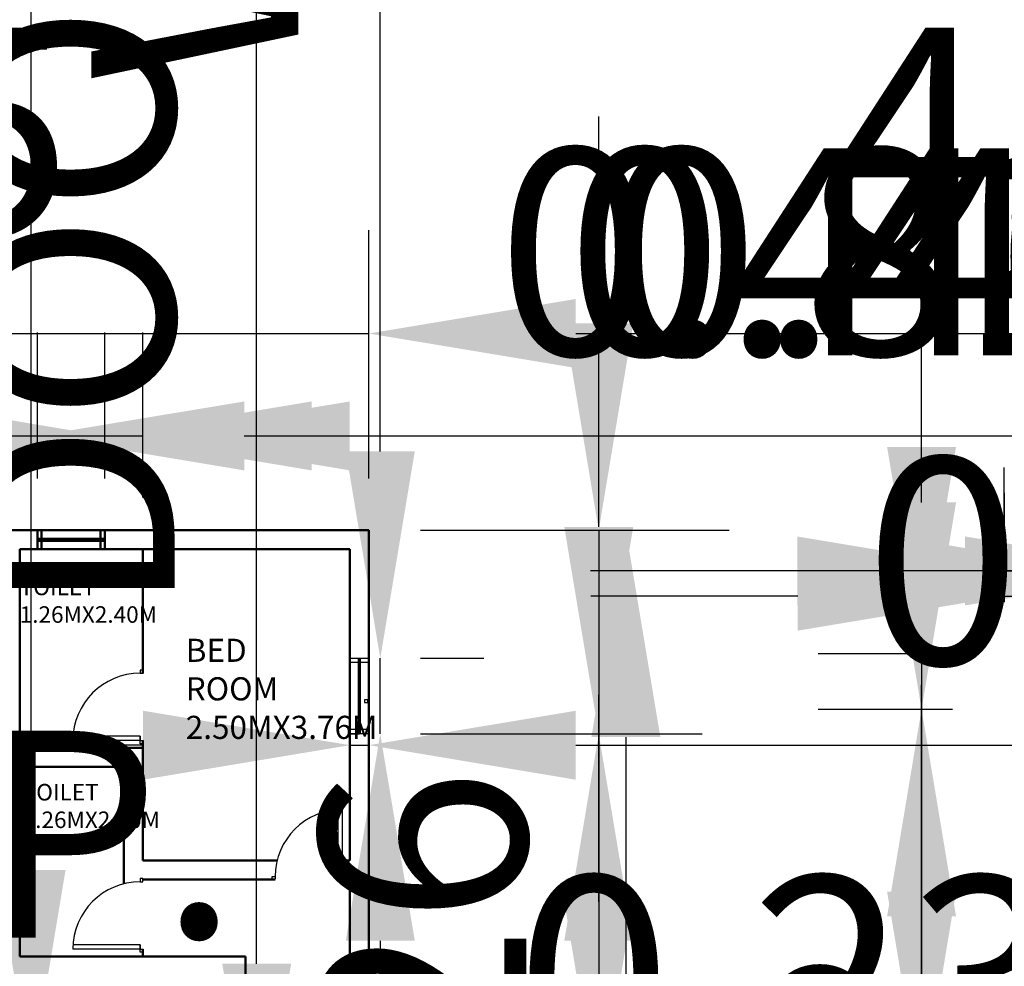
# Model space of a CAD drawing. Units: metres. Extents: x 782 to 1487, y 1262 to 7446.
# Tile 17 of 25: x 828.19 to 840.09, y 1302.06 to 1313.5. Entities that reach past the tile are written whole.
import ezdxf

# ---------------------------------------------------------------- set-up
doc = ezdxf.new("R2010")
doc.units = ezdxf.units.M
for name, color, linetype, lineweight in [('A-ANNO-DIMS', 2, 'Continuous', 18), ('A-AREA-IDEN', 3, 'Continuous', 18), ('A-DOOR', 4, 'Continuous', 25), ('A-GLAZ', 4, 'Continuous', 25), ('A-WALL', 7, 'Continuous', 50)]:
    doc.layers.add(name, color=color, linetype=linetype, lineweight=lineweight)
doc.styles.get("Standard").update_dxf_attribs({"font": 'arial.ttf'})
doc.dimstyles.new('ISO-25', dxfattribs={"dimtxt": 2.5, "dimasz": 2.5, "dimexe": 1.25, "dimexo": 0.625, "dimtad": 1, "dimtxsty": 'Standard', "dimcen": 2.5, "dimadec": 0, "dimazin": 0, "dimtfac": 1, "dimtmove": 0, "dimatfit": 3, "dimfxl": 1, "dimarcsym": 0})

# ---------------------------------------------------------------- blocks, each defined once
blk = doc.blocks.new('*D5')
at = {"layer": 'A-ANNO-DIMS', "color": 0, "lineweight": -2, "transparency": 16777216}
for p, q in [((812.13, 1307.952), (812.13, 1310.955)), ((816.58, 1307.952), (816.58, 1310.955)), ((809.63, 1309.705), (807.13, 1309.705)), ((812.13, 1309.705), (816.58, 1309.705)), ((819.08, 1309.705), (829.443, 1309.705))]:
    blk.add_line(p, q, dxfattribs=at)
at = {"layer": 'A-ANNO-DIMS', "color": 0, "transparency": 16777216}
for points in [[(809.63, 1310.122), (809.63, 1309.289), (812.13, 1309.705)], [(819.08, 1310.122), (819.08, 1309.289), (816.58, 1309.705)]]:
    blk.add_solid(points, dxfattribs=at)
at = {"layer": 'Defpoints', "color": 0, "transparency": 16777216}
for p in [(816.58, 1309.705), (812.13, 1307.327), (816.58, 1307.327)]:
    blk.add_point(p, dxfattribs=at)
at = {"layer": 'A-ANNO-DIMS', "color": 0, "transparency": 16777216, "insert": (825.512, 1311.828), "char_height": 2.5, "attachment_point": 5}
blk.add_mtext('4,45', dxfattribs=at)
blk = doc.blocks.new('*D6')
at = {"layer": 'A-ANNO-DIMS', "color": 0, "lineweight": -2, "transparency": 16777216}
for p, q in [((833.037, 1307.327), (836.768, 1307.327)), ((835.518, 1304.827), (835.518, 1295.567)), ((833.037, 1293.067), (836.768, 1293.067))]:
    blk.add_line(p, q, dxfattribs=at)
at = {"layer": 'A-ANNO-DIMS', "color": 0, "transparency": 16777216}
for points in [[(835.102, 1304.827), (835.935, 1304.827), (835.518, 1307.327)], [(835.102, 1295.567), (835.935, 1295.567), (835.518, 1293.067)]]:
    blk.add_solid(points, dxfattribs=at)
at = {"layer": 'Defpoints', "color": 0, "transparency": 16777216}
for p in [(832.412, 1307.327), (832.412, 1293.067), (835.518, 1293.067)]:
    blk.add_point(p, dxfattribs=at)
at = {"layer": 'A-ANNO-DIMS', "color": 0, "transparency": 16777216, "insert": (833.391, 1300.197), "char_height": 2.5, "attachment_point": 5, "rotation": 90}
blk.add_mtext('14,26', dxfattribs=at)
blk = doc.blocks.new('*D7')
at = {"layer": 'A-ANNO-DIMS', "color": 0, "lineweight": -2, "transparency": 16777216}
for p, q in [((827.962, 1307.952), (827.962, 1310.955)), ((832.412, 1307.952), (832.412, 1310.955)), ((825.462, 1309.705), (822.962, 1309.705)), ((827.962, 1309.705), (832.412, 1309.705)), ((834.912, 1309.705), (845.276, 1309.705))]:
    blk.add_line(p, q, dxfattribs=at)
at = {"layer": 'A-ANNO-DIMS', "color": 0, "transparency": 16777216}
for points in [[(825.462, 1310.122), (825.462, 1309.289), (827.962, 1309.705)], [(834.912, 1310.122), (834.912, 1309.289), (832.412, 1309.705)]]:
    blk.add_solid(points, dxfattribs=at)
at = {"layer": 'Defpoints', "color": 0, "transparency": 16777216}
for p in [(832.412, 1309.705), (827.962, 1307.327), (832.412, 1307.327)]:
    blk.add_point(p, dxfattribs=at)
at = {"layer": 'A-ANNO-DIMS', "color": 0, "transparency": 16777216, "insert": (841.344, 1311.828), "char_height": 2.5, "attachment_point": 5}
blk.add_mtext('4,45', dxfattribs=at)
blk = doc.blocks.new('*D9')
at = {"layer": 'A-ANNO-DIMS', "color": 0, "lineweight": -2, "transparency": 16777216}
for p, q in [((840.095, 1306.46), (840.095, 1307.78)), ((844.185, 1306.46), (844.185, 1307.78)), ((837.595, 1306.53), (835.095, 1306.53)), ((840.095, 1306.53), (844.185, 1306.53)), ((846.685, 1306.53), (857.034, 1306.53))]:
    blk.add_line(p, q, dxfattribs=at)
at = {"layer": 'A-ANNO-DIMS', "color": 0, "transparency": 16777216}
for points in [[(837.595, 1306.947), (837.595, 1306.114), (840.095, 1306.53)], [(846.685, 1306.947), (846.685, 1306.114), (844.185, 1306.53)]]:
    blk.add_solid(points, dxfattribs=at)
at = {"layer": 'Defpoints', "color": 0, "transparency": 16777216}
for p in [(844.185, 1306.53), (840.095, 1305.835), (844.185, 1305.835)]:
    blk.add_point(p, dxfattribs=at)
at = {"layer": 'A-ANNO-DIMS', "color": 0, "transparency": 16777216, "insert": (853.11, 1308.658), "char_height": 2.5, "attachment_point": 5}
blk.add_mtext('4,09', dxfattribs=at)
blk = doc.blocks.new('DOOR-810')
for p, q in [((0.813, 0.089), (0, 0.089)), ((0.813, 0.038), (0.813, 0.089))]:
    blk.add_line(p, q)
for points in [[(0.813, 0.851), (0.846, 0.851), (0.846, 0.89), (0.813, 0.89)], [(0.813, 0.038), (0.847, 0.038), (0.847, 0), (0.813, 0)]]:
    blk.add_lwpolyline(points, close=True)
blk.add_lwpolyline([(0.813, 0.089), (0.813, 0.038), (0, 0.038)])
blk.add_arc((0.813, 0.038), 0.813, 90, 180)
blk = doc.blocks.new('DOOR-810-C')
for p, q in [((0.801, 0.034), (0.801, 0.847)), ((0.851, 0.034), (0.801, 0.034))]:
    blk.add_line(p, q)
blk.add_lwpolyline([(0.801, 0.034), (0.851, 0.034), (0.851, 0.847)])
for points in [[(0.039, 0.034), (0.039, 0.002), (0, 0.002), (0, 0.034)], [(0.851, 0.034), (0.851, 0), (0.889, 0), (0.889, 0.034)]]:
    blk.add_lwpolyline(points, close=True)
blk.add_arc((0.851, 0.034), 0.813, 90, 180)
blk = doc.blocks.new('WIN-900-B')
for p, q in [((0, 0), (0, 0.914)), ((0, 0.914), (0.23, 0.914)), ((0.23, 0.863), (0, 0.863)), ((0.103, 0), (0.103, 0.914)), ((0.115, 0), (0.115, 0.914)), ((0.128, 0), (0.128, 0.914)), ((0.23, 0.914), (0.23, 0)), ((0.23, 0.914), (0.23, 0.863)), ((0.23, 0.051), (0, 0.051)), ((0.23, 0), (0.23, 0.051)), ((0.23, 0), (0, 0)), ((0, 0), (0.115, 0))]:
    blk.add_line(p, q)
blk.add_lwpolyline([(0.215, 0.379), (0.215, 0.412), (0.176, 0.412), (0.176, 0.379)], close=True)
blk = doc.blocks.new('*D20')
at = {"layer": 'A-ANNO-DIMS', "color": 0, "lineweight": -2, "transparency": 16777216}
for p, q in [((831.056, 1302.088), (831.056, 1337.678)), ((831.056, 1298.698), (831.056, 1299.588)), ((831.548, 1299.588), (832.306, 1299.588)), ((831.548, 1298.698), (832.306, 1298.698)), ((831.056, 1296.198), (831.056, 1293.698))]:
    blk.add_line(p, q, dxfattribs=at)
at = {"layer": 'A-ANNO-DIMS', "color": 0, "transparency": 16777216}
for points in [[(830.64, 1302.088), (831.473, 1302.088), (831.056, 1299.588)], [(830.64, 1296.198), (831.473, 1296.198), (831.056, 1298.698)]]:
    blk.add_solid(points, dxfattribs=at)
at = {"layer": 'Defpoints', "color": 0, "transparency": 16777216}
for p in [(830.923, 1299.588), (831.056, 1299.588), (830.923, 1298.698)]:
    blk.add_point(p, dxfattribs=at)
at = {"layer": 'A-ANNO-DIMS', "color": 0, "transparency": 16777216, "insert": (829.138, 1321.133), "char_height": 2.5, "attachment_point": 5, "rotation": 90}
blk.add_mtext('DOOR D1 0.89 TYP.', dxfattribs=at)
blk = doc.blocks.new('*D21')
at = {"layer": 'A-ANNO-DIMS', "color": 0, "lineweight": -2, "transparency": 16777216}
for p, q in [((827.576, 1298.565), (825.076, 1298.565)), ((830.076, 1298.565), (830.923, 1298.565)), ((833.423, 1298.565), (852.255, 1298.565)), ((830.076, 1298.073), (830.076, 1297.315)), ((830.923, 1298.073), (830.923, 1297.315))]:
    blk.add_line(p, q, dxfattribs=at)
at = {"layer": 'A-ANNO-DIMS', "color": 0, "transparency": 16777216}
for points in [[(827.576, 1298.981), (827.576, 1298.148), (830.076, 1298.565)], [(833.423, 1298.981), (833.423, 1298.148), (830.923, 1298.565)]]:
    blk.add_solid(points, dxfattribs=at)
at = {"layer": 'Defpoints', "color": 0, "transparency": 16777216}
for p in [(830.076, 1298.698), (830.923, 1298.698), (830.923, 1298.565)]:
    blk.add_point(p, dxfattribs=at)
at = {"layer": 'A-ANNO-DIMS', "color": 0, "transparency": 16777216, "insert": (844.089, 1300.466), "char_height": 2.5, "attachment_point": 5}
blk.add_mtext('0.85 TYP.', dxfattribs=at)
blk = doc.blocks.new('*D24')
at = {"layer": 'A-ANNO-DIMS', "color": 0, "lineweight": -2, "transparency": 16777216}
for p, q in [((811.209, 1294.423), (808.709, 1294.423)), ((813.709, 1294.423), (814.559, 1294.423)), ((817.059, 1294.423), (852.649, 1294.423)), ((813.709, 1293.926), (813.709, 1293.173)), ((814.559, 1293.926), (814.559, 1293.173))]:
    blk.add_line(p, q, dxfattribs=at)
at = {"layer": 'A-ANNO-DIMS', "color": 0, "transparency": 16777216}
for points in [[(811.209, 1294.84), (811.209, 1294.006), (813.709, 1294.423)], [(817.059, 1294.84), (817.059, 1294.006), (814.559, 1294.423)]]:
    blk.add_solid(points, dxfattribs=at)
at = {"layer": 'Defpoints', "color": 0, "transparency": 16777216}
for p in [(813.709, 1294.551), (814.559, 1294.551), (814.559, 1294.423)]:
    blk.add_point(p, dxfattribs=at)
at = {"layer": 'A-ANNO-DIMS', "color": 0, "transparency": 16777216, "insert": (836.104, 1296.342), "char_height": 2.5, "attachment_point": 5}
blk.add_mtext('DOOR D2 0.85 TYP.', dxfattribs=at)
blk = doc.blocks.new('*D26')
at = {"layer": 'A-ANNO-DIMS', "color": 0, "lineweight": -2, "transparency": 16777216}
for p, q in [((828.33, 1303.223), (828.33, 1342.718)), ((828.33, 1299.809), (828.33, 1300.723)), ((828.818, 1300.723), (829.58, 1300.723)), ((828.818, 1299.809), (829.58, 1299.809)), ((828.33, 1297.309), (828.33, 1294.809))]:
    blk.add_line(p, q, dxfattribs=at)
at = {"layer": 'A-ANNO-DIMS', "color": 0, "transparency": 16777216}
for points in [[(827.913, 1303.223), (828.747, 1303.223), (828.33, 1300.723)], [(827.913, 1297.309), (828.747, 1297.309), (828.33, 1299.809)]]:
    blk.add_solid(points, dxfattribs=at)
at = {"layer": 'Defpoints', "color": 0, "transparency": 16777216}
for p in [(828.193, 1300.723), (828.33, 1300.723), (828.193, 1299.809)]:
    blk.add_point(p, dxfattribs=at)
at = {"layer": 'A-ANNO-DIMS', "color": 0, "transparency": 16777216, "insert": (826.412, 1324.22), "char_height": 2.5, "attachment_point": 5, "rotation": 90}
blk.add_mtext('WINDOW W 0.91 TYP.', dxfattribs=at)
blk = doc.blocks.new('*D27')
at = {"layer": 'A-ANNO-DIMS', "color": 0, "lineweight": -2, "transparency": 16777216}
for p, q in [((825.463, 1299.672), (822.963, 1299.672)), ((827.963, 1299.672), (828.193, 1299.672)), ((830.693, 1299.672), (849.525, 1299.672)), ((827.963, 1299.184), (827.963, 1298.422)), ((828.193, 1299.184), (828.193, 1298.422))]:
    blk.add_line(p, q, dxfattribs=at)
at = {"layer": 'A-ANNO-DIMS', "color": 0, "transparency": 16777216}
for points in [[(825.463, 1300.088), (825.463, 1299.255), (827.963, 1299.672)], [(830.693, 1300.088), (830.693, 1299.255), (828.193, 1299.672)]]:
    blk.add_solid(points, dxfattribs=at)
at = {"layer": 'Defpoints', "color": 0, "transparency": 16777216}
for p in [(827.963, 1299.809), (828.193, 1299.809), (828.193, 1299.672)]:
    blk.add_point(p, dxfattribs=at)
at = {"layer": 'A-ANNO-DIMS', "color": 0, "transparency": 16777216, "insert": (841.359, 1301.574), "char_height": 2.5, "attachment_point": 5}
blk.add_mtext('0.23 TYP.', dxfattribs=at)
blk = doc.blocks.new('*D28')
at = {"layer": 'A-ANNO-DIMS', "color": 0, "lineweight": -2, "transparency": 16777216}
for p, q in [((832.55, 1308.281), (832.55, 1349.718)), ((832.55, 1304.867), (832.55, 1305.781)), ((833.038, 1305.781), (833.8, 1305.781)), ((833.038, 1304.867), (833.8, 1304.867)), ((832.55, 1302.367), (832.55, 1299.867))]:
    blk.add_line(p, q, dxfattribs=at)
at = {"layer": 'A-ANNO-DIMS', "color": 0, "transparency": 16777216}
for points in [[(832.134, 1308.281), (832.967, 1308.281), (832.55, 1305.781)], [(832.134, 1302.367), (832.967, 1302.367), (832.55, 1304.867)]]:
    blk.add_solid(points, dxfattribs=at)
at = {"layer": 'Defpoints', "color": 0, "transparency": 16777216}
for p in [(832.413, 1305.781), (832.55, 1305.781), (832.413, 1304.867)]:
    blk.add_point(p, dxfattribs=at)
at = {"layer": 'A-ANNO-DIMS', "color": 0, "transparency": 16777216, "insert": (830.632, 1330.25), "char_height": 2.5, "attachment_point": 5, "rotation": 90}
blk.add_mtext('WINDOW W1 0.91 TYP.', dxfattribs=at)
blk = doc.blocks.new('*D29')
at = {"layer": 'A-ANNO-DIMS', "color": 0, "lineweight": -2, "transparency": 16777216}
for p, q in [((829.683, 1304.73), (827.183, 1304.73)), ((832.183, 1304.73), (832.413, 1304.73)), ((834.913, 1304.73), (853.745, 1304.73)), ((832.183, 1304.242), (832.183, 1303.48)), ((832.413, 1304.242), (832.413, 1303.48))]:
    blk.add_line(p, q, dxfattribs=at)
at = {"layer": 'A-ANNO-DIMS', "color": 0, "transparency": 16777216}
for points in [[(829.683, 1305.146), (829.683, 1304.313), (832.183, 1304.73)], [(834.913, 1305.146), (834.913, 1304.313), (832.413, 1304.73)]]:
    blk.add_solid(points, dxfattribs=at)
at = {"layer": 'Defpoints', "color": 0, "transparency": 16777216}
for p in [(832.183, 1304.867), (832.413, 1304.867), (832.413, 1304.73)]:
    blk.add_point(p, dxfattribs=at)
at = {"layer": 'A-ANNO-DIMS', "color": 0, "transparency": 16777216, "insert": (845.579, 1306.632), "char_height": 2.5, "attachment_point": 5}
blk.add_mtext('0.23 TYP.', dxfattribs=at)
blk = doc.blocks.new('*D30')
at = {"layer": 'A-ANNO-DIMS', "color": 0, "lineweight": -2, "transparency": 16777216}
for p, q in [((792.059, 1301.411), (789.559, 1301.411)), ((794.559, 1301.411), (794.946, 1301.411)), ((797.446, 1301.411), (832.354, 1301.411)), ((794.559, 1300.844), (794.559, 1300.161)), ((794.946, 1300.844), (794.946, 1300.161))]:
    blk.add_line(p, q, dxfattribs=at)
at = {"layer": 'A-ANNO-DIMS', "color": 0, "transparency": 16777216}
for points in [[(792.059, 1301.827), (792.059, 1300.994), (794.559, 1301.411)], [(797.446, 1301.827), (797.446, 1300.994), (794.946, 1301.411)]]:
    blk.add_solid(points, dxfattribs=at)
at = {"layer": 'Defpoints', "color": 0, "transparency": 16777216}
for p in [(794.559, 1301.469), (794.946, 1301.469), (794.946, 1301.411)]:
    blk.add_point(p, dxfattribs=at)
at = {"layer": 'A-ANNO-DIMS', "color": 0, "transparency": 16777216, "insert": (816.15, 1303.33), "char_height": 2.5, "attachment_point": 5}
blk.add_mtext('COLUMN 0.39 TYP.', dxfattribs=at)
blk = doc.blocks.new('*D87')
at = {"layer": 'A-ANNO-DIMS', "color": 0, "lineweight": -2, "transparency": 16777216}
for p, q in [((835.19, 1309.827), (835.19, 1312.327)), ((833.037, 1307.327), (836.44, 1307.327)), ((835.19, 1307.327), (835.19, 1304.867)), ((833.038, 1304.867), (836.44, 1304.867)), ((835.19, 1302.367), (835.19, 1292.082))]:
    blk.add_line(p, q, dxfattribs=at)
at = {"layer": 'A-ANNO-DIMS', "color": 0, "transparency": 16777216}
for points in [[(834.774, 1309.827), (835.607, 1309.827), (835.19, 1307.327)], [(834.774, 1302.367), (835.607, 1302.367), (835.19, 1304.867)]]:
    blk.add_solid(points, dxfattribs=at)
at = {"layer": 'Defpoints', "color": 0, "transparency": 16777216}
for p in [(832.412, 1307.327), (832.413, 1304.867), (835.19, 1304.867)]:
    blk.add_point(p, dxfattribs=at)
at = {"layer": 'A-ANNO-DIMS', "color": 0, "transparency": 16777216, "insert": (833.289, 1295.974), "char_height": 2.5, "attachment_point": 5, "rotation": 90}
blk.add_mtext('2.46', dxfattribs=at)
blk = doc.blocks.new('*D88')
at = {"layer": 'A-ANNO-DIMS', "color": 0, "lineweight": -2, "transparency": 16777216}
for p, q in [((835.19, 1307.367), (835.19, 1309.867)), ((833.038, 1304.867), (836.44, 1304.867)), ((835.19, 1304.867), (835.19, 1300.338)), ((833.038, 1300.338), (836.44, 1300.338)), ((835.19, 1297.838), (835.19, 1285.546))]:
    blk.add_line(p, q, dxfattribs=at)
at = {"layer": 'A-ANNO-DIMS', "color": 0, "transparency": 16777216}
for points in [[(834.774, 1307.367), (835.607, 1307.367), (835.19, 1304.867)], [(834.774, 1297.838), (835.607, 1297.838), (835.19, 1300.338)]]:
    blk.add_solid(points, dxfattribs=at)
at = {"layer": 'Defpoints', "color": 0, "transparency": 16777216}
for p in [(832.413, 1304.867), (832.413, 1300.338), (835.19, 1300.338)]:
    blk.add_point(p, dxfattribs=at)
at = {"layer": 'A-ANNO-DIMS', "color": 0, "transparency": 16777216, "insert": (833.289, 1290.442), "char_height": 2.5, "attachment_point": 5, "rotation": 90}
blk.add_mtext('4.529', dxfattribs=at)
blk = doc.blocks.new('*D89')
at = {"layer": 'A-ANNO-DIMS', "color": 0, "lineweight": -2, "transparency": 16777216}
for p, q in [((835.19, 1302.838), (835.19, 1305.338)), ((833.038, 1300.338), (836.44, 1300.338)), ((835.19, 1300.338), (835.19, 1296.196)), ((833.037, 1296.196), (836.44, 1296.196)), ((835.19, 1293.696), (835.19, 1281.435))]:
    blk.add_line(p, q, dxfattribs=at)
at = {"layer": 'A-ANNO-DIMS', "color": 0, "transparency": 16777216}
for points in [[(834.774, 1302.838), (835.607, 1302.838), (835.19, 1300.338)], [(834.774, 1293.696), (835.607, 1293.696), (835.19, 1296.196)]]:
    blk.add_solid(points, dxfattribs=at)
at = {"layer": 'Defpoints', "color": 0, "transparency": 16777216}
for p in [(832.413, 1300.338), (832.412, 1296.196), (835.19, 1296.196)]:
    blk.add_point(p, dxfattribs=at)
at = {"layer": 'A-ANNO-DIMS', "color": 0, "transparency": 16777216, "insert": (833.31, 1286.315), "char_height": 2.5, "attachment_point": 5, "rotation": 90}
blk.add_mtext('4.142', dxfattribs=at)
blk = doc.blocks.new('*D94')
at = {"layer": 'A-ANNO-DIMS', "color": 0, "lineweight": -2, "transparency": 16777216}
for p, q in [((827.962, 1307.952), (827.962, 1309.718)), ((828.406, 1307.953), (828.406, 1309.718)), ((825.462, 1308.468), (822.962, 1308.468)), ((827.962, 1308.468), (828.406, 1308.468)), ((830.906, 1308.468), (841.139, 1308.468))]:
    blk.add_line(p, q, dxfattribs=at)
at = {"layer": 'A-ANNO-DIMS', "color": 0, "transparency": 16777216}
for points in [[(825.462, 1308.884), (825.462, 1308.051), (827.962, 1308.468)], [(830.906, 1308.884), (830.906, 1308.051), (828.406, 1308.468)]]:
    blk.add_solid(points, dxfattribs=at)
at = {"layer": 'Defpoints', "color": 0, "transparency": 16777216}
for p in [(828.406, 1308.468), (827.962, 1307.327), (828.406, 1307.328)]:
    blk.add_point(p, dxfattribs=at)
at = {"layer": 'A-ANNO-DIMS', "color": 0, "transparency": 16777216, "insert": (837.273, 1310.369), "char_height": 2.5, "attachment_point": 5}
blk.add_mtext('0.44', dxfattribs=at)
blk = doc.blocks.new('*D95')
at = {"layer": 'A-ANNO-DIMS', "color": 0, "lineweight": -2, "transparency": 16777216}
for p, q in [((828.406, 1307.953), (828.406, 1309.718)), ((829.22, 1307.953), (829.22, 1309.718)), ((825.906, 1308.468), (823.406, 1308.468)), ((828.406, 1308.468), (829.22, 1308.468)), ((831.72, 1308.468), (843.896, 1308.468))]:
    blk.add_line(p, q, dxfattribs=at)
at = {"layer": 'A-ANNO-DIMS', "color": 0, "transparency": 16777216}
for points in [[(825.906, 1308.884), (825.906, 1308.051), (828.406, 1308.468)], [(831.72, 1308.884), (831.72, 1308.051), (829.22, 1308.468)]]:
    blk.add_solid(points, dxfattribs=at)
at = {"layer": 'Defpoints', "color": 0, "transparency": 16777216}
for p in [(829.22, 1308.468), (828.406, 1307.328), (829.22, 1307.328)]:
    blk.add_point(p, dxfattribs=at)
at = {"layer": 'A-ANNO-DIMS', "color": 0, "transparency": 16777216, "insert": (839.058, 1310.369), "char_height": 2.5, "attachment_point": 5}
blk.add_mtext('0.814', dxfattribs=at)
blk = doc.blocks.new('*D96')
at = {"layer": 'A-ANNO-DIMS', "color": 0, "lineweight": -2, "transparency": 16777216}
for p, q in [((829.22, 1307.953), (829.22, 1309.718)), ((829.682, 1307.722), (829.682, 1309.718)), ((826.72, 1308.468), (824.22, 1308.468)), ((829.22, 1308.468), (829.682, 1308.468)), ((832.182, 1308.468), (842.425, 1308.468))]:
    blk.add_line(p, q, dxfattribs=at)
at = {"layer": 'A-ANNO-DIMS', "color": 0, "transparency": 16777216}
for points in [[(826.72, 1308.884), (826.72, 1308.051), (829.22, 1308.468)], [(832.182, 1308.884), (832.182, 1308.051), (829.682, 1308.468)]]:
    blk.add_solid(points, dxfattribs=at)
at = {"layer": 'Defpoints', "color": 0, "transparency": 16777216}
for p in [(829.682, 1308.468), (829.22, 1307.328), (829.682, 1307.097)]:
    blk.add_point(p, dxfattribs=at)
at = {"layer": 'A-ANNO-DIMS', "color": 0, "transparency": 16777216, "insert": (838.554, 1310.369), "char_height": 2.5, "attachment_point": 5}
blk.add_mtext('0.46', dxfattribs=at)
blk = doc.blocks.new('*D101')
at = {"layer": 'A-ANNO-DIMS', "color": 0, "lineweight": -2, "transparency": 16777216}
for p, q in [((840.091, 1306.46), (840.091, 1308.085)), ((841.28, 1306.46), (841.28, 1308.085)), ((837.591, 1306.835), (835.091, 1306.835)), ((840.091, 1306.835), (841.28, 1306.835)), ((843.78, 1306.835), (853.794, 1306.835))]:
    blk.add_line(p, q, dxfattribs=at)
at = {"layer": 'A-ANNO-DIMS', "color": 0, "transparency": 16777216}
for points in [[(837.591, 1307.252), (837.591, 1306.419), (840.091, 1306.835)], [(843.78, 1307.252), (843.78, 1306.419), (841.28, 1306.835)]]:
    blk.add_solid(points, dxfattribs=at)
at = {"layer": 'Defpoints', "color": 0, "transparency": 16777216}
for p in [(841.28, 1306.835), (840.091, 1305.835), (841.28, 1305.835)]:
    blk.add_point(p, dxfattribs=at)
at = {"layer": 'A-ANNO-DIMS', "color": 0, "transparency": 16777216, "insert": (850.037, 1308.737), "char_height": 2.5, "attachment_point": 5}
blk.add_mtext('1.19', dxfattribs=at)
blk = doc.blocks.new('*D102')
at = {"layer": 'A-ANNO-DIMS', "color": 0, "lineweight": -2, "transparency": 16777216}
for p, q in [((841.28, 1306.46), (841.28, 1308.085)), ((842.118, 1306.46), (842.118, 1308.085)), ((838.78, 1306.835), (836.28, 1306.835)), ((841.28, 1306.835), (842.118, 1306.835)), ((844.618, 1306.835), (856.81, 1306.835))]:
    blk.add_line(p, q, dxfattribs=at)
at = {"layer": 'A-ANNO-DIMS', "color": 0, "transparency": 16777216}
for points in [[(838.78, 1307.252), (838.78, 1306.419), (841.28, 1306.835)], [(844.618, 1307.252), (844.618, 1306.419), (842.118, 1306.835)]]:
    blk.add_solid(points, dxfattribs=at)
at = {"layer": 'Defpoints', "color": 0, "transparency": 16777216}
for p in [(842.118, 1306.835), (841.28, 1305.835), (842.118, 1305.835)]:
    blk.add_point(p, dxfattribs=at)
at = {"layer": 'A-ANNO-DIMS', "color": 0, "transparency": 16777216, "insert": (851.964, 1308.738), "char_height": 2.5, "attachment_point": 5}
blk.add_mtext('0.838', dxfattribs=at)
blk = doc.blocks.new('*D103')
at = {"layer": 'A-ANNO-DIMS', "color": 0, "lineweight": -2, "transparency": 16777216}
for p, q in [((842.118, 1306.46), (842.118, 1308.085)), ((842.956, 1306.46), (842.956, 1308.085)), ((839.618, 1306.835), (837.118, 1306.835)), ((842.118, 1306.835), (842.956, 1306.835)), ((845.456, 1306.835), (857.648, 1306.835))]:
    blk.add_line(p, q, dxfattribs=at)
at = {"layer": 'A-ANNO-DIMS', "color": 0, "transparency": 16777216}
for points in [[(839.618, 1307.252), (839.618, 1306.419), (842.118, 1306.835)], [(845.456, 1307.252), (845.456, 1306.419), (842.956, 1306.835)]]:
    blk.add_solid(points, dxfattribs=at)
at = {"layer": 'Defpoints', "color": 0, "transparency": 16777216}
for p in [(842.956, 1306.835), (842.118, 1305.835), (842.956, 1305.835)]:
    blk.add_point(p, dxfattribs=at)
at = {"layer": 'A-ANNO-DIMS', "color": 0, "transparency": 16777216, "insert": (852.802, 1308.738), "char_height": 2.5, "attachment_point": 5}
blk.add_mtext('0.838', dxfattribs=at)
blk = doc.blocks.new('*D104')
at = {"layer": 'A-ANNO-DIMS', "color": 0, "lineweight": -2, "transparency": 16777216}
for p, q in [((842.956, 1306.46), (842.956, 1308.085)), ((844.185, 1306.46), (844.185, 1308.085)), ((840.456, 1306.835), (837.956, 1306.835)), ((842.956, 1306.835), (844.185, 1306.835)), ((846.685, 1306.835), (856.693, 1306.835))]:
    blk.add_line(p, q, dxfattribs=at)
at = {"layer": 'A-ANNO-DIMS', "color": 0, "transparency": 16777216}
for points in [[(840.456, 1307.252), (840.456, 1306.419), (842.956, 1306.835)], [(846.685, 1307.252), (846.685, 1306.419), (844.185, 1306.835)]]:
    blk.add_solid(points, dxfattribs=at)
at = {"layer": 'Defpoints', "color": 0, "transparency": 16777216}
for p in [(844.185, 1306.835), (842.956, 1305.835), (844.185, 1305.835)]:
    blk.add_point(p, dxfattribs=at)
at = {"layer": 'A-ANNO-DIMS', "color": 0, "transparency": 16777216, "insert": (852.939, 1308.738), "char_height": 2.5, "attachment_point": 5}
blk.add_mtext('1.23', dxfattribs=at)
blk = doc.blocks.new('*D109')
at = {"layer": 'A-ANNO-DIMS', "color": 0, "lineweight": -2, "transparency": 16777216}
for p, q in [((839.091, 1308.335), (839.091, 1310.835)), ((839.466, 1305.835), (837.841, 1305.835)), ((839.091, 1305.835), (839.091, 1305.163)), ((839.466, 1305.163), (837.841, 1305.163)), ((839.091, 1302.663), (839.091, 1290.503))]:
    blk.add_line(p, q, dxfattribs=at)
at = {"layer": 'A-ANNO-DIMS', "color": 0, "transparency": 16777216}
for points in [[(838.675, 1308.335), (839.508, 1308.335), (839.091, 1305.835)], [(838.675, 1302.663), (839.508, 1302.663), (839.091, 1305.163)]]:
    blk.add_solid(points, dxfattribs=at)
at = {"layer": 'Defpoints', "color": 0, "transparency": 16777216}
for p in [(840.091, 1305.835), (839.091, 1305.163), (840.091, 1305.163)]:
    blk.add_point(p, dxfattribs=at)
at = {"layer": 'A-ANNO-DIMS', "color": 0, "transparency": 16777216, "insert": (837.19, 1295.333), "char_height": 2.5, "attachment_point": 5, "rotation": 90}
blk.add_mtext('0.672', dxfattribs=at)
blk = doc.blocks.new('*D110')
at = {"layer": 'A-ANNO-DIMS', "color": 0, "lineweight": -2, "transparency": 16777216}
for p, q in [((839.091, 1307.663), (839.091, 1310.163)), ((839.466, 1305.163), (837.841, 1305.163)), ((839.091, 1305.163), (839.091, 1300.459)), ((839.466, 1300.459), (837.841, 1300.459)), ((839.091, 1297.959), (839.091, 1285.683))]:
    blk.add_line(p, q, dxfattribs=at)
at = {"layer": 'A-ANNO-DIMS', "color": 0, "transparency": 16777216}
for points in [[(838.675, 1307.663), (839.508, 1307.663), (839.091, 1305.163)], [(838.675, 1297.959), (839.508, 1297.959), (839.091, 1300.459)]]:
    blk.add_solid(points, dxfattribs=at)
at = {"layer": 'Defpoints', "color": 0, "transparency": 16777216}
for p in [(840.091, 1305.163), (839.091, 1300.459), (840.091, 1300.459)]:
    blk.add_point(p, dxfattribs=at)
at = {"layer": 'A-ANNO-DIMS', "color": 0, "transparency": 16777216, "insert": (837.19, 1290.571), "char_height": 2.5, "attachment_point": 5, "rotation": 90}
blk.add_mtext('4.704', dxfattribs=at)
blk = doc.blocks.new('*D111')
at = {"layer": 'A-ANNO-DIMS', "color": 0, "lineweight": -2, "transparency": 16777216}
for p, q in [((839.091, 1302.959), (839.091, 1305.459)), ((839.466, 1300.459), (837.841, 1300.459)), ((839.091, 1300.459), (839.091, 1299.115)), ((839.466, 1299.115), (837.841, 1299.115)), ((839.091, 1296.615), (839.091, 1284.675))]:
    blk.add_line(p, q, dxfattribs=at)
at = {"layer": 'A-ANNO-DIMS', "color": 0, "transparency": 16777216}
for points in [[(838.675, 1302.959), (839.508, 1302.959), (839.091, 1300.459)], [(838.675, 1296.615), (839.508, 1296.615), (839.091, 1299.115)]]:
    blk.add_solid(points, dxfattribs=at)
at = {"layer": 'Defpoints', "color": 0, "transparency": 16777216}
for p in [(840.091, 1300.459), (839.091, 1299.115), (840.091, 1299.115)]:
    blk.add_point(p, dxfattribs=at)
at = {"layer": 'A-ANNO-DIMS', "color": 0, "transparency": 16777216, "insert": (837.189, 1289.395), "char_height": 2.5, "attachment_point": 5, "rotation": 90}
blk.add_mtext('1.344', dxfattribs=at)
blk = doc.blocks.new('*D112')
at = {"layer": 'A-ANNO-DIMS', "color": 0, "lineweight": -2, "transparency": 16777216}
for p, q in [((839.091, 1301.615), (839.091, 1304.115)), ((839.466, 1299.115), (837.841, 1299.115)), ((839.091, 1299.115), (839.091, 1293.067)), ((839.466, 1293.067), (837.841, 1293.067)), ((839.091, 1290.567), (839.091, 1278.362))]:
    blk.add_line(p, q, dxfattribs=at)
at = {"layer": 'A-ANNO-DIMS', "color": 0, "transparency": 16777216}
for points in [[(838.675, 1301.615), (839.508, 1301.615), (839.091, 1299.115)], [(838.675, 1290.567), (839.508, 1290.567), (839.091, 1293.067)]]:
    blk.add_solid(points, dxfattribs=at)
at = {"layer": 'Defpoints', "color": 0, "transparency": 16777216}
for p in [(840.091, 1299.115), (839.091, 1293.067), (840.091, 1293.067)]:
    blk.add_point(p, dxfattribs=at)
at = {"layer": 'A-ANNO-DIMS', "color": 0, "transparency": 16777216, "insert": (837.19, 1283.215), "char_height": 2.5, "attachment_point": 5, "rotation": 90}
blk.add_mtext('6.048', dxfattribs=at)

msp = doc.modelspace()

# ---------------------------------------------------------------- linework, layer by layer
at = {"layer": 'A-WALL'}
for p, q in [((827.9625, 1307.3274), (829.4525, 1307.3274)), ((828.4057, 1307.3276), (829.2197, 1307.3276)), ((828.4057, 1307.0976), (828.4057, 1307.3276)), ((828.4057, 1307.3276), (828.4057, 1307.2126)), ((828.4565, 1307.0976), (828.4565, 1307.3276)), ((829.1689, 1307.0976), (829.1689, 1307.3276)), ((829.2197, 1307.3276), (829.2197, 1307.0976)), ((829.4525, 1307.3274), (832.4125, 1307.3274)), ((832.4125, 1307.3274), (832.4125, 1303.3374)), ((828.4057, 1307.2253), (829.2197, 1307.2253)), ((828.4057, 1307.2126), (829.2197, 1307.2126)), ((828.1925, 1304.6974), (828.1925, 1307.0974)), ((828.1925, 1307.0974), (832.1825, 1307.0974)), ((828.4057, 1307.1999), (829.2197, 1307.1999)), ((829.2197, 1307.0976), (828.4057, 1307.0976)), ((828.4057, 1307.0976), (828.4565, 1307.0976)), ((829.2197, 1307.0976), (829.1689, 1307.0976)), ((829.6825, 1307.0974), (829.6825, 1305.5981)), ((829.6825, 1307.0974), (832.1825, 1307.0974)), ((829.6825, 1305.5981), (829.6825, 1307.0974)), ((832.1825, 1307.0974), (832.1825, 1303.3374)), ((829.6825, 1304.786), (829.6825, 1304.6974)), ((829.6825, 1303.3374), (829.6825, 1304.786)), ((829.6825, 1304.6974), (829.6825, 1304.7482)), ((828.1925, 1304.6974), (829.4525, 1304.6974)), ((829.4525, 1304.6974), (829.6825, 1304.6974)), ((828.1925, 1302.1774), (828.1925, 1304.4674)), ((828.1925, 1304.4674), (829.4525, 1304.4674)), ((828.1925, 1304.4674), (829.4525, 1304.4674)), ((829.4525, 1304.4674), (829.4525, 1303.0548)), ((829.4525, 1303.3374), (829.4525, 1304.4674)), ((829.4525, 1304.4674), (829.6825, 1304.4674)), ((829.6825, 1304.4674), (829.6825, 1304.4166)), ((831.3051, 1303.3374), (829.6825, 1303.3374)), ((832.1825, 1303.3374), (832.0938, 1303.3374)), ((832.4125, 1303.3374), (832.4125, 1293.0674)), ((831.2818, 1303.1074), (829.6825, 1303.1074)), ((832.1825, 1303.1074), (832.0938, 1303.1074)), ((832.1825, 1303.1074), (832.1317, 1303.1074)), ((832.1825, 1303.1074), (832.1825, 1298.6474)), ((829.6825, 1302.266), (829.6825, 1302.1774)), ((829.6825, 1302.1774), (829.6825, 1302.2282)), ((828.1925, 1302.1774), (830.9225, 1302.1774)), ((830.9225, 1302.1774), (830.9225, 1299.5481))]:
    msp.add_line(p, q, dxfattribs=at)

# ---------------------------------------------------------------- block references
at = {"layer": 'A-DOOR'}
for name, p in [('DOOR-810', (828.836, 1304.748)), ('DOOR-810-C', (831.242, 1303.107)), ('DOOR-810', (828.836, 1302.228))]:
    msp.add_blockref(name, p, dxfattribs=at)
at = {"layer": 'A-GLAZ'}
msp.add_blockref('WIN-900-B', (832.183, 1304.867), dxfattribs=at)

# ---------------------------------------------------------------- texts
at = {"layer": 'A-AREA-IDEN', "attachment_point": 1}
for s, width, gutter_width, insert, char_height in [('\\P{\\H0.4x;TOILET\\P1.26MX2.40M}', 1.153085, 12.5, (828.1925, 1307.5758), 0.5), ('BED ROOM\\P2.50MX3.76M', 0.64421, 6.9836, (830.199, 1306.0163), 0.279342), ('\\P{\\H0.4x;TOILET\\P1.26MX2.40M}', 1.153085, 12.5, (828.2284, 1305.0951), 0.5)]:
    msp.add_mtext_dynamic_manual_height_columns(s, width=width, gutter_width=gutter_width, heights=[0], dxfattribs=dict(at, insert=insert, char_height=char_height))

# ---------------------------------------------------------------- dimensions: what is measured, and where the dimension line sits
at = {"layer": 'A-ANNO-DIMS'}
for base, p1, p2, text, picture, middle in [((832.5503, 1305.7809), (832.4132, 1304.8669), (832.4132, 1305.7809), 'WINDOW W1 <> TYP.', '*D28', (830.6318, 1330.2497)), ((828.3302, 1300.7228), (828.1931, 1299.8088), (828.1931, 1300.7228), 'WINDOW W <> TYP.', '*D26', (826.4117, 1324.2204)), ((831.0564, 1299.5877), (830.923, 1298.6982), (830.923, 1299.5877), 'DOOR D1 <> TYP.', '*D20', (829.138, 1321.1327))]:
    dim = msp.add_linear_dim(base=base, p1=p1, p2=p2, angle=90, text=text, dimstyle='ISO-25', override={"dimdec": 2, "dimlfac": 1, "dimrnd": 0, "dimzin": 0, "dimdsep": 46, "dimlunit": 2}, dxfattribs=at)
    dim.commit()
    dim.dimension.update_dxf_attribs({"geometry": picture, "text_midpoint": middle})
for base, p1, p2, override, picture, middle in [((816.58, 1309.7054), (812.13, 1307.3274), (816.58, 1307.3274), {"dimclrd": 0, "dimclre": 0, "dimclrt": 0}, '*D5', (825.5116, 1311.8277)), ((832.4125, 1309.7054), (827.9625, 1307.3274), (832.4125, 1307.3274), {"dimclrd": 0, "dimclre": 0, "dimclrt": 0}, '*D7', (841.3441, 1311.8277)), ((828.4057, 1308.4676), (827.9625, 1307.3274), (828.4057, 1307.3276), {"dimdec": 2, "dimlfac": 1, "dimrnd": 0, "dimzin": 0, "dimdsep": 46, "dimlunit": 2}, '*D94', (837.2725, 1310.369)), ((829.2197, 1308.4676), (828.4057, 1307.3276), (829.2197, 1307.3276), {"dimdec": 3, "dimlfac": 1, "dimrnd": 0, "dimzin": 0, "dimdsep": 46, "dimlunit": 2}, '*D95', (839.0577, 1310.369)), ((829.6825, 1308.4676), (829.2197, 1307.3276), (829.6825, 1307.0974), {"dimdec": 2, "dimlfac": 1, "dimrnd": 0, "dimzin": 0, "dimdsep": 46, "dimlunit": 2}, '*D96', (838.5536, 1310.369)), ((841.2801, 1306.8353), (840.0913, 1305.8353), (841.2801, 1305.8353), {"dimdec": 2, "dimlfac": 1, "dimrnd": 0, "dimzin": 0, "dimdsep": 46, "dimlunit": 2}, '*D101', (850.037, 1308.7367)), ((842.1182, 1306.8353), (841.2801, 1305.8353), (842.1182, 1305.8353), {"dimdec": 3, "dimlfac": 1, "dimrnd": 0, "dimzin": 0, "dimdsep": 46, "dimlunit": 2}, '*D102', (851.9639, 1308.7376)), ((842.9563, 1306.8353), (842.1182, 1305.8353), (842.9563, 1305.8353), {"dimdec": 3, "dimlfac": 1, "dimrnd": 0, "dimzin": 0, "dimdsep": 46, "dimlunit": 2}, '*D103', (852.802, 1308.7376)), ((844.1849, 1306.8353), (842.9563, 1305.8353), (844.1849, 1305.8353), {"dimdec": 2, "dimlfac": 1, "dimrnd": 0, "dimzin": 0, "dimdsep": 46, "dimlunit": 2}, '*D104', (852.9391, 1308.7376)), ((844.1849, 1306.5303), (840.0949, 1305.8353), (844.1849, 1305.8353), {"dimclrd": 0, "dimclre": 0, "dimclrt": 0}, '*D9', (853.1097, 1308.6577))]:
    dim = msp.add_linear_dim(base=base, p1=p1, p2=p2, dimstyle='ISO-25', override=override, dxfattribs=at)
    dim.commit()
    dim.dimension.update_dxf_attribs({"geometry": picture, "text_midpoint": middle})
for base, p1, p2, override, picture, middle in [((835.1905, 1304.8669), (832.4125, 1307.3274), (832.4132, 1304.8669), {"dimdec": 2, "dimlfac": 1, "dimrnd": 0, "dimzin": 0, "dimdsep": 46, "dimlunit": 2}, '*D87', (833.289, 1295.9745)), ((839.0913, 1305.1633), (840.0913, 1305.8353), (840.0913, 1305.1633), {"dimdec": 3, "dimlfac": 1, "dimrnd": 0, "dimzin": 0, "dimdsep": 46, "dimlunit": 2}, '*D109', (837.1899, 1295.333)), ((839.0913, 1300.4593), (840.0913, 1305.1633), (840.0913, 1300.4593), {"dimdec": 3, "dimlfac": 1, "dimrnd": 0, "dimzin": 0, "dimdsep": 46, "dimlunit": 2}, '*D110', (837.1899, 1290.571)), ((835.1905, 1300.3378), (832.4132, 1304.8669), (832.4131, 1300.3378), {"dimdec": 3, "dimlfac": 1, "dimrnd": 0, "dimzin": 0, "dimdsep": 46, "dimlunit": 2}, '*D88', (833.289, 1290.4419)), ((835.5183, 1293.0674), (832.4125, 1307.3274), (832.4125, 1293.0674), {"dimclrd": 0, "dimclre": 0, "dimclrt": 0}, '*D6', (833.3909, 1300.1974)), ((839.0913, 1299.1153), (840.0913, 1300.4593), (840.0913, 1299.1153), {"dimdec": 3, "dimlfac": 1, "dimrnd": 0, "dimzin": 0, "dimdsep": 46, "dimlunit": 2}, '*D111', (837.189, 1289.395)), ((835.1905, 1296.196), (832.4131, 1300.3378), (832.4125, 1296.196), {"dimdec": 3, "dimlfac": 1, "dimrnd": 0, "dimzin": 0, "dimdsep": 46, "dimlunit": 2}, '*D89', (833.3103, 1286.3153)), ((839.0913, 1293.0674), (840.0913, 1299.1153), (840.0913, 1293.0674), {"dimdec": 3, "dimlfac": 1, "dimrnd": 0, "dimzin": 0, "dimdsep": 46, "dimlunit": 2}, '*D112', (837.1899, 1283.2149))]:
    dim = msp.add_linear_dim(base=base, p1=p1, p2=p2, angle=90, dimstyle='ISO-25', override=override, dxfattribs=at)
    dim.commit()
    dim.dimension.update_dxf_attribs({"geometry": picture, "text_midpoint": middle})
for base, p1, p2, text, picture, middle in [((832.4132, 1304.7298), (832.1832, 1304.8669), (832.4132, 1304.8669), '<> TYP.', '*D29', (845.5791, 1306.6321)), ((794.9459, 1301.4107), (794.559, 1301.4687), (794.9459, 1301.4687), 'COLUMN <> TYP.', '*D30', (816.1499, 1303.33)), ((828.1931, 1299.6717), (827.9631, 1299.8088), (828.1931, 1299.8088), '<> TYP.', '*D27', (841.359, 1301.574)), ((814.5592, 1294.4231), (813.7086, 1294.5507), (814.5592, 1294.5507), 'DOOR D2 <> TYP.', '*D24', (836.1042, 1296.3416)), ((830.923, 1298.5648), (830.0763, 1298.6982), (830.923, 1298.6982), '<> TYP.', '*D21', (844.0889, 1300.4662))]:
    dim = msp.add_linear_dim(base=base, p1=p1, p2=p2, text=text, dimstyle='ISO-25', override={"dimdec": 2, "dimlfac": 1, "dimrnd": 0, "dimzin": 0, "dimdsep": 46, "dimlunit": 2}, dxfattribs=at)
    dim.commit()
    dim.dimension.update_dxf_attribs({"geometry": picture, "text_midpoint": middle})

doc.saveas('drawing.dxf')
